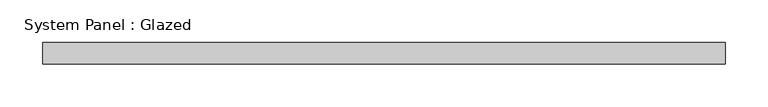
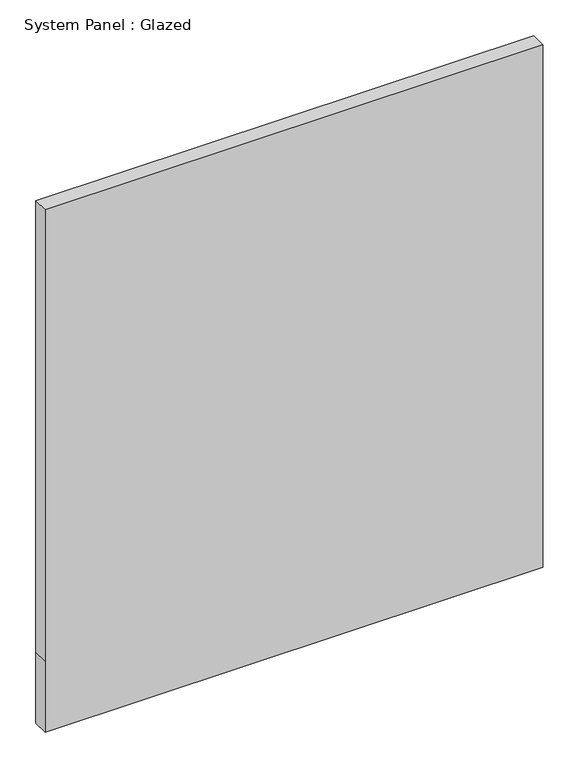
"""IFC4 building model written with IfcOpenShell, lengths in millimetres: plate geometry, System Panel : Glazed."""

from ifc_helpers import new_model, si_unit, frame, origin, place, context, project, spatial, polyline, outline, extrude, source, transform, mapped, element, save


def system_panel_glazed_21a2a3f6(model_context):
    return source(origin(), model_context, "Body", "SweptSolid", [
        extrude(outline(polyline([(0.0, -400.05), (0.0, 400.05), (120.65, 400.05), (887.8244987, 400.05), (887.8244987, -400.05), (120.65, -400.05), (0.0, -400.05)])), frame((0.0, 19.05, 0.0), z_axis=(0.0, 1.0, 0.0), x_axis=(0.0, 0.0, 1.0)), (0.0, 0.0, 1.0), 25.4),
    ])


if __name__ == "__main__":
    model = new_model("IFC4")
    model_context = context("Model", 3, world=origin())
    ifc_project = project(units=[si_unit("LENGTHUNIT", "METRE", prefix="MILLI")], contexts=[model_context])
    site = spatial("IfcSite", under=ifc_project)
    building = spatial("IfcBuilding", under=site)
    placement = place(None, origin())
    system_panel_glazed_shape = system_panel_glazed_21a2a3f6(model_context)
    element("IfcPlate", 1, ObjectType="System Panel : Glazed", at=placement, inside=building, context=model_context, shape_type="MappedRepresentation", body=[
        mapped(system_panel_glazed_shape, transform((0.0, 0.0, 0.0), x_axis=(1.0, 0.0, 0.0), y_axis=(0.0, 1.0, 0.0), z_axis=(0.0, 0.0, 1.0))),
    ])
    save(model, "model.ifc")

# Revit data of these elements
# Type "System Panel : Glazed"
#   Construction Type Id = "GSP4R"
#   Analytic Construction = "1/8 in Pilkington single glazing"
#   Visual Light Transmittance = 0.9
#   Solar Heat Gain Coefficient = 0.86
#   Heat Transfer Coefficient (U) = 1.18115 BTU/(h·ft²·°F)
#   Define Thermal Properties by = 1
# Element 1 (IfcPlate, "System Panel : Glazed")
#   Materials on its faces: "Glass"
# Materials
#   "Glass": class "Glass", colour RGB 0 128 192, transparency 0.75, Description = "Soda Lime Glass", Cost = 0
